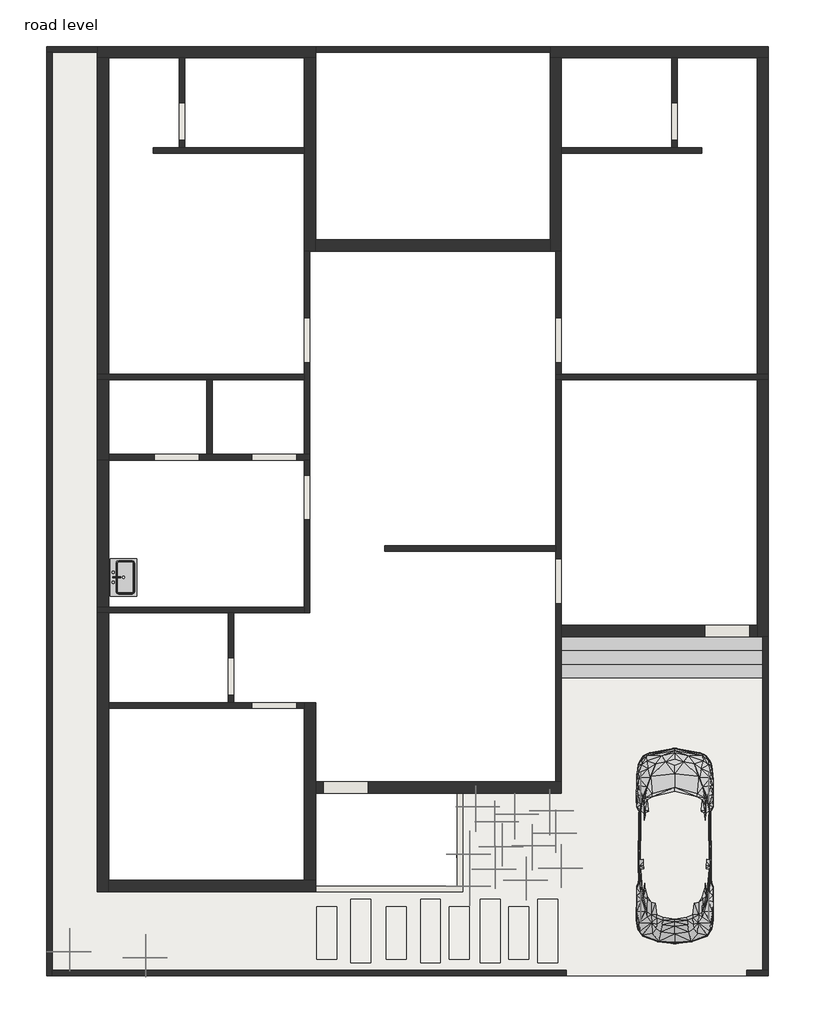
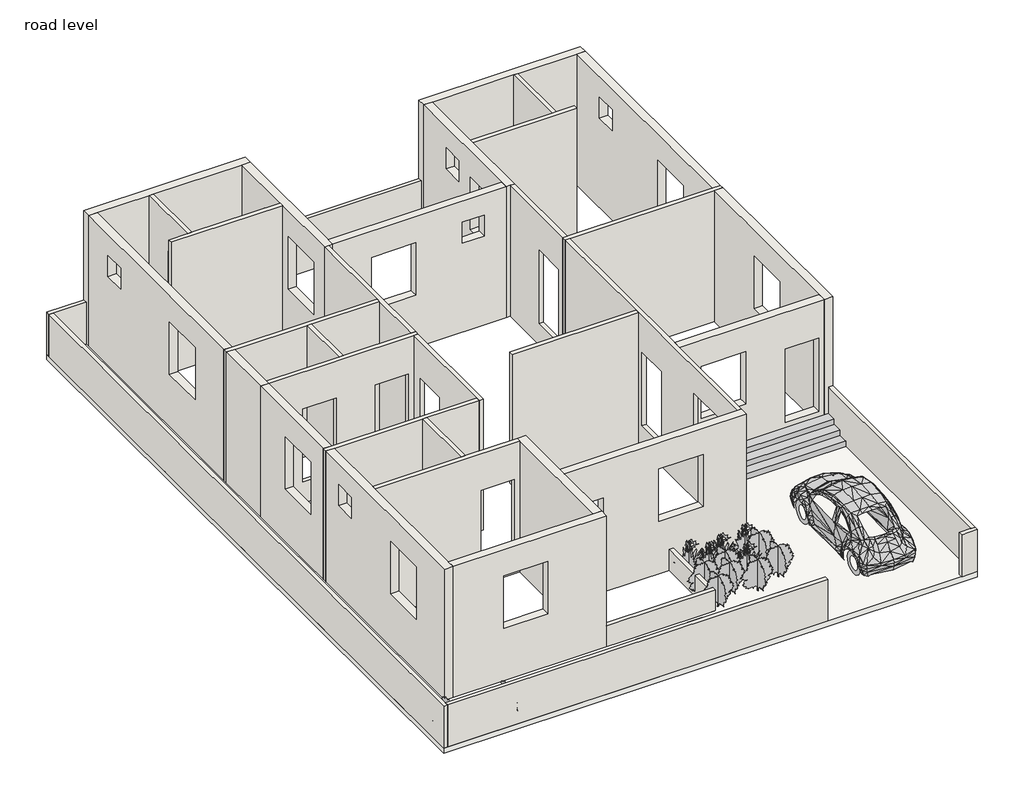
# One storey: 39 walls, 14 geographic elements, 2 slabs, 1 flow terminal, 1 furniture element, 1 proxy.
"""IFC4 building model written with IfcOpenShell, lengths in millimetres."""

from ifc_helpers import new_model, si_unit, frame, origin, origin_with_axes, place, context, project, spatial, polyline, outline, extrude, faceted_brep, transform, mapped, element, save
from components import rpc_beetle_rpc_beetle_31f8b51e, flow_terminal_4d548711, casework_15_casework_15_947a4ada, rpc_plant_tropical_55f6ff97, rpc_plant_tropical_jungle_flame_3_9c4808c2

model = new_model("IFC4")

# Units and contexts
model_context = context("Model", 3, world=origin())
ifc_project = project(units=[si_unit("LENGTHUNIT", "METRE", prefix="MILLI")], contexts=[model_context])

# Site, building, storey
site = spatial("IfcSite", under=ifc_project)
building = spatial("IfcBuilding", under=site)
storey = spatial("IfcBuildingStorey", under=building, Name="road level", Elevation=0.0)

# Proxy
placement = place(None, origin())
rpc_beetle_rpc_beetle_shape = rpc_beetle_rpc_beetle_31f8b51e(model_context)
element("IfcBuildingElementProxy", 1, Name="RPC Beetle : RPC Beetle", ObjectType="RPC Beetle : RPC Beetle", at=placement, inside=storey, context=model_context, shape_type="MappedRepresentation", body=[
    mapped(rpc_beetle_rpc_beetle_shape, transform((12469.3923267, -477.4503076, 0.0), x_axis=(1.0, 0.0, 0.0), y_axis=(0.0, 1.0, 0.0), z_axis=(0.0, 0.0, 1.0))),
])

# Flow terminal
flow_terminal_shape = flow_terminal_4d548711(model_context)
element("IfcFlowTerminal", 2, ObjectType="Sink Kitchen-Single : 30\" x 21\"", at=placement, inside=storey, context=model_context, shape_type="MappedRepresentation", body=[
    mapped(flow_terminal_shape, transform((1244.9377278, 6212.4604519, 0.0), x_axis=(0.0, 1.0, 0.0), y_axis=(-1.0, 0.0, 0.0), z_axis=(0.0, 0.0, 1.0))),
])

# Furniture
casework_15_casework_15_shape = casework_15_casework_15_947a4ada(model_context)
element("IfcFurniture", 3, ObjectType="Casework 15 : Casework 15", at=placement, inside=storey, context=model_context, shape_type="MappedRepresentation", body=[
    mapped(casework_15_casework_15_shape, transform((0.0, 0.0, 0.0), x_axis=(1.0, 0.0, 0.0), y_axis=(0.0, 1.0, 0.0), z_axis=(0.0, 0.0, 1.0))),
])

# Geographic elements
rpc_plant_tropical_shape = rpc_plant_tropical_55f6ff97(model_context)
element("IfcGeographicElement", 4, ObjectType="RPC Plant - Tropical", at=placement, inside=storey, context=model_context, shape_type="MappedRepresentation", body=[
    mapped(rpc_plant_tropical_shape, transform((8418.0923267, 1554.5496924, 0.0), x_axis=(1.0, 0.0, 0.0), y_axis=(0.0, 1.0, 0.0), z_axis=(0.0, 0.0, 1.0))),
])
element("IfcGeographicElement", 5, ObjectType="RPC Plant - Tropical", at=placement, inside=storey, context=model_context, shape_type="MappedRepresentation", body=[
    mapped(rpc_plant_tropical_shape, transform((9205.4923267, 1402.1496924, 0.0), x_axis=(1.0, 0.0, 0.0), y_axis=(0.0, 1.0, 0.0), z_axis=(0.0, 0.0, 1.0))),
])
element("IfcGeographicElement", 6, ObjectType="RPC Plant - Tropical", at=placement, inside=storey, context=model_context, shape_type="MappedRepresentation", body=[
    mapped(rpc_plant_tropical_shape, transform((9916.6923267, 1478.3496924, 0.0), x_axis=(1.0, 0.0, 0.0), y_axis=(0.0, 1.0, 0.0), z_axis=(0.0, 0.0, 1.0))),
])
element("IfcGeographicElement", 7, ObjectType="RPC Plant - Tropical", at=placement, inside=storey, context=model_context, shape_type="MappedRepresentation", body=[
    mapped(rpc_plant_tropical_shape, transform((8799.0923267, 1249.7496924, 0.0), x_axis=(1.0, 0.0, 0.0), y_axis=(0.0, 1.0, 0.0), z_axis=(0.0, 0.0, 1.0))),
])
element("IfcGeographicElement", 8, ObjectType="RPC Plant - Tropical", at=placement, inside=storey, context=model_context, shape_type="MappedRepresentation", body=[
    mapped(rpc_plant_tropical_shape, transform((9561.0923267, 767.1496924, 0.0), x_axis=(1.0, 0.0, 0.0), y_axis=(0.0, 1.0, 0.0), z_axis=(0.0, 0.0, 1.0))),
])
rpc_plant_tropical_jungle_flame_3_shape = rpc_plant_tropical_jungle_flame_3_9c4808c2(model_context)
element("IfcGeographicElement", 9, ObjectType="RPC Plant - Tropical : Jungle Flame - 3'", at=placement, inside=storey, context=model_context, shape_type="MappedRepresentation", body=[
    mapped(rpc_plant_tropical_jungle_flame_3_shape, transform((8291.0923267, 589.3496924, 0.0), x_axis=(1.0, 0.0, 0.0), y_axis=(0.0, 1.0, 0.0), z_axis=(0.0, 0.0, 1.0))),
])
element("IfcGeographicElement", 10, ObjectType="RPC Plant - Tropical : Jungle Flame - 3'", at=placement, inside=storey, context=model_context, shape_type="MappedRepresentation", body=[
    mapped(rpc_plant_tropical_jungle_flame_3_shape, transform((8951.4923267, 741.7496924, 0.0), x_axis=(1.0, 0.0, 0.0), y_axis=(0.0, 1.0, 0.0), z_axis=(0.0, 0.0, 1.0))),
])
element("IfcGeographicElement", 11, ObjectType="RPC Plant - Tropical : Jungle Flame - 3'", at=placement, inside=storey, context=model_context, shape_type="MappedRepresentation", body=[
    mapped(rpc_plant_tropical_jungle_flame_3_shape, transform((10157.9923267, 309.9496924, 0.0), x_axis=(1.0, 0.0, 0.0), y_axis=(0.0, 1.0, 0.0), z_axis=(0.0, 0.0, 1.0))),
])
element("IfcGeographicElement", 12, ObjectType="RPC Plant - Tropical : Jungle Flame - 3'", at=placement, inside=storey, context=model_context, shape_type="MappedRepresentation", body=[
    mapped(rpc_plant_tropical_jungle_flame_3_shape, transform((10043.6923267, 1021.1496924, 0.0), x_axis=(1.0, 0.0, 0.0), y_axis=(0.0, 1.0, 0.0), z_axis=(0.0, 0.0, 1.0))),
])
element("IfcGeographicElement", 13, ObjectType="RPC Plant - Tropical : Jungle Flame - 3'", at=placement, inside=storey, context=model_context, shape_type="MappedRepresentation", body=[
    mapped(rpc_plant_tropical_jungle_flame_3_shape, transform((9446.9910318, 55.9496924, 0.0), x_axis=(1.0, 0.0, 0.0), y_axis=(0.0, 1.0, 0.0), z_axis=(0.0, 0.0, 1.0))),
])
element("IfcGeographicElement", 14, ObjectType="RPC Plant - Tropical : Jungle Flame - 3'", at=placement, inside=storey, context=model_context, shape_type="MappedRepresentation", body=[
    mapped(rpc_plant_tropical_jungle_flame_3_shape, transform((8291.0923267, -58.3503076, 0.0), x_axis=(1.0, 0.0, 0.0), y_axis=(0.0, 1.0, 0.0), z_axis=(0.0, 0.0, 1.0))),
])
element("IfcGeographicElement", 15, ObjectType="RPC Plant - Tropical : Jungle Flame - 3'", at=placement, inside=storey, context=model_context, shape_type="MappedRepresentation", body=[
    mapped(rpc_plant_tropical_jungle_flame_3_shape, transform((8807.0822913, 284.5496924, 0.0), x_axis=(1.0, 0.0, 0.0), y_axis=(0.0, 1.0, 0.0), z_axis=(0.0, 0.0, 1.0))),
])
element("IfcGeographicElement", 16, ObjectType="RPC Plant - Tropical : Jungle Flame - 3'", at=placement, inside=storey, context=model_context, shape_type="MappedRepresentation", body=[
    mapped(rpc_plant_tropical_jungle_flame_3_shape, transform((150.3923267, -1391.8503076, 0.0), x_axis=(1.0, 0.0, 0.0), y_axis=(0.0, 1.0, 0.0), z_axis=(0.0, 0.0, 1.0))),
])
element("IfcGeographicElement", 17, ObjectType="RPC Plant - Tropical : Jungle Flame - 3'", at=placement, inside=storey, context=model_context, shape_type="MappedRepresentation", body=[
    mapped(rpc_plant_tropical_jungle_flame_3_shape, transform((1699.7923267, -1518.8503076, 0.0), x_axis=(1.0, 0.0, 0.0), y_axis=(0.0, 1.0, 0.0), z_axis=(0.0, 0.0, 1.0))),
])

# Slabs
element("IfcSlab", 18, at=placement, inside=storey, context=model_context, shape_type="SweptSolid", body=[
    extrude(outline(polyline([(5586.9696389, -1544.2503076), (5180.5696389, -1544.2503076), (5180.5696389, -477.4503076), (5586.9696389, -477.4503076), (5586.9696389, -1544.2503076)])), frame((0.0, 0.0, -50.8), z_axis=(0.0, 0.0, 1.0), x_axis=(1.0, 0.0, 0.0)), (0.0, 0.0, 1.0), 101.6),
    extrude(outline(polyline([(6276.4251133, -1620.4503076), (5870.0251133, -1620.4503076), (5870.0251133, -325.0503076), (6276.4251133, -325.0503076), (6276.4251133, -1620.4503076)])), frame((0.0, 0.0, -50.8), z_axis=(0.0, 0.0, 1.0), x_axis=(1.0, 0.0, 0.0)), (0.0, 0.0, 1.0), 101.6),
    extrude(outline(polyline([(6999.06314, -1544.2503076), (6592.66314, -1544.2503076), (6592.66314, -477.4503076), (6999.06314, -477.4503076), (6999.06314, -1544.2503076)])), frame((0.0, 0.0, -50.8), z_axis=(0.0, 0.0, 1.0), x_axis=(1.0, 0.0, 0.0)), (0.0, 0.0, 1.0), 101.6),
    extrude(outline(polyline([(7696.9670249, -1620.4503076), (7290.5670249, -1620.4503076), (7290.5670249, -325.0503076), (7696.9670249, -325.0503076), (7696.9670249, -1620.4503076)])), frame((0.0, 0.0, -50.8), z_axis=(0.0, 0.0, 1.0), x_axis=(1.0, 0.0, 0.0)), (0.0, 0.0, 1.0), 101.6),
    extrude(outline(polyline([(8277.6567255, -1544.2503076), (7871.2567255, -1544.2503076), (7871.2567255, -477.4503076), (8277.6567255, -477.4503076), (8277.6567255, -1544.2503076)])), frame((0.0, 0.0, -50.8), z_axis=(0.0, 0.0, 1.0), x_axis=(1.0, 0.0, 0.0)), (0.0, 0.0, 1.0), 101.6),
    extrude(outline(polyline([(8916.1156077, -1620.4503076), (8509.7156077, -1620.4503076), (8509.7156077, -325.0503076), (8916.1156077, -325.0503076), (8916.1156077, -1620.4503076)])), frame((0.0, 0.0, -50.8), z_axis=(0.0, 0.0, 1.0), x_axis=(1.0, 0.0, 0.0)), (0.0, 0.0, 1.0), 101.6),
    extrude(outline(polyline([(9492.8822913, -1544.2503076), (9086.4822913, -1544.2503076), (9086.4822913, -477.4503076), (9492.8822913, -477.4503076), (9492.8822913, -1544.2503076)])), frame((0.0, 0.0, -50.8), z_axis=(0.0, 0.0, 1.0), x_axis=(1.0, 0.0, 0.0)), (0.0, 0.0, 1.0), 101.6),
    extrude(outline(polyline([(10081.9910318, -1620.4503076), (9675.5910318, -1620.4503076), (9675.5910318, -325.0503076), (10081.9910318, -325.0503076), (10081.9910318, -1620.4503076)])), frame((0.0, 0.0, -50.8), z_axis=(0.0, 0.0, 1.0), x_axis=(1.0, 0.0, 0.0)), (0.0, 0.0, 1.0), 101.6),
])
element("IfcSlab", 19, at=placement, inside=storey, context=model_context, shape_type="SweptSolid", body=[
    extrude(outline(polyline([(709.1923267, 17035.8496924), (709.1923267, -172.6503076), (8151.3923267, -172.6503076), (8151.3923267, 1833.9496924), (10157.9923267, 1833.9496924), (10157.9923267, 5021.6496924), (14374.3923267, 5021.6496924), (14374.3923267, -1887.1503076), (-319.5076733, -1887.1503076), (-319.5076733, 17035.8496924), (709.1923267, 17035.8496924)])), frame((0.0, 0.0, -152.4), z_axis=(0.0, 0.0, 1.0), x_axis=(1.0, 0.0, 0.0)), (0.0, 0.0, 1.0), 152.4),
])

# Walls
element("IfcWall", 20, at=placement, inside=storey, context=model_context, shape_type="Brep", body=[
    faceted_brep([(709.1923267, 16807.2496924, 3810.0), (709.1923267, 16807.2496924, 0.0), (937.7923267, 16807.2496924, 0.0), (2372.8923267, 16807.2496924, 0.0), (2487.1923267, 16807.2496924, 0.0), (4925.5923267, 16807.2496924, 0.0), (5154.1923267, 16807.2496924, 0.0), (5154.1923267, 16807.2496924, 3810.0), (4925.5923267, 16807.2496924, 3810.0), (2487.1923267, 16807.2496924, 3810.0), (2372.8923267, 16807.2496924, 3810.0), (937.7923267, 16807.2496924, 3810.0), (709.1923267, 17035.8496924, 0.0), (709.1923267, 17035.8496924, 1219.2), (709.1923267, 17035.8496924, 3810.0), (5154.1923267, 17035.8496924, 3810.0), (5154.1923267, 17035.8496924, 1524.0), (5154.1923267, 17035.8496924, 0.0), (709.1923267, 16921.5496924, 0.0), (5154.1923267, 16921.5496924, 0.0)], [[[0, 1, 2, 3, 4, 5, 6, 7, 8, 9, 10, 11]], [[12, 13, 14, 15, 16, 17]], [[6, 5, 4, 3, 2, 1, 18, 12, 17, 19]], [[0, 11, 10, 9, 8, 7, 15, 14]], [[6, 19, 17, 16, 15, 7]], [[0, 14, 13, 12, 18, 1]]]),
])
element("IfcWall", 21, at=placement, inside=storey, context=model_context, shape_type="Brep", body=[
    faceted_brep([(4925.5923267, 16807.2496924, 3810.0), (4925.5923267, 16807.2496924, 0.0), (4925.5923267, 14978.4496924, 0.0), (4925.5923267, 14864.1496924, 0.0), (4925.5923267, 12870.2496924, 0.0), (4925.5923267, 12870.2496924, 3810.0), (4925.5923267, 14864.1496924, 3810.0), (4925.5923267, 14978.4496924, 3810.0), (4925.5923267, 13390.9496924, 3048.0), (4925.5923267, 13390.9496924, 1524.0), (4925.5923267, 14610.1496924, 1524.0), (4925.5923267, 14610.1496924, 3048.0), (4925.5923267, 15130.8496924, 3200.4), (4925.5923267, 15130.8496924, 2590.8), (4925.5923267, 15740.4496924, 2590.8), (4925.5923267, 15740.4496924, 3200.4), (5154.1923267, 16807.2496924, 0.0), (5154.1923267, 16807.2496924, 3810.0), (5154.1923267, 13098.8496924, 3810.0), (5154.1923267, 12870.2496924, 3810.0), (5154.1923267, 12870.2496924, 0.0), (5154.1923267, 13098.8496924, 0.0), (5154.1923267, 13390.9496924, 3048.0), (5154.1923267, 14610.1496924, 3048.0), (5154.1923267, 14610.1496924, 1524.0), (5154.1923267, 13390.9496924, 1524.0), (5154.1923267, 15130.8496924, 3200.4), (5154.1923267, 15740.4496924, 3200.4), (5154.1923267, 15740.4496924, 2590.8), (5154.1923267, 15130.8496924, 2590.8), (5039.8923267, 12870.2496924, 0.0), (5039.8923267, 12870.2496924, 3810.0)], [[[0, 1, 2, 3, 4, 5, 6, 7], [8, 9, 10, 11], [12, 13, 14, 15]], [[16, 17, 18, 19, 20, 21], [22, 23, 24, 25], [26, 27, 28, 29]], [[4, 3, 2, 1, 16, 21, 20, 30]], [[0, 7, 6, 5, 31, 19, 18, 17]], [[5, 4, 30, 20, 19, 31]], [[9, 8, 22, 25]], [[10, 9, 25, 24]], [[11, 10, 24, 23]], [[8, 11, 23, 22]], [[13, 12, 26, 29]], [[14, 13, 29, 28]], [[15, 14, 28, 27]], [[12, 15, 27, 26]], [[0, 17, 16, 1]]]),
])
element("IfcWall", 22, at=placement, inside=storey, context=model_context, shape_type="Brep", body=[
    faceted_brep([(4925.5923267, 14978.4496924, 0.0), (2487.1923267, 14978.4496924, 0.0), (2372.8923267, 14978.4496924, 0.0), (1852.1923267, 14978.4496924, 0.0), (1852.1923267, 14978.4496924, 3810.0), (2372.8923267, 14978.4496924, 3810.0), (2487.1923267, 14978.4496924, 3810.0), (4925.5923267, 14978.4496924, 3810.0), (4925.5923267, 14864.1496924, 0.0), (4925.5923267, 14864.1496924, 3810.0), (1852.1923267, 14864.1496924, 3810.0), (1852.1923267, 14864.1496924, 0.0)], [[[0, 1, 2, 3, 4, 5, 6, 7]], [[8, 9, 10, 11]], [[3, 2, 1, 0, 8, 11]], [[4, 3, 11, 10]], [[7, 6, 5, 4, 10, 9]], [[0, 7, 9, 8]]]),
])
element("IfcWall", 23, at=placement, inside=storey, context=model_context, shape_type="Brep", body=[
    faceted_brep([(4925.5923267, 10368.3496924, 0.0), (937.7923267, 10368.3496924, 0.0), (709.1923267, 10368.3496924, 0.0), (709.1923267, 10368.3496924, 3810.0), (937.7923267, 10368.3496924, 3810.0), (4925.5923267, 10368.3496924, 3810.0), (4925.5923267, 10254.0496924, 0.0), (4925.5923267, 10254.0496924, 3810.0), (3052.3423267, 10254.0496924, 3810.0), (2938.0423267, 10254.0496924, 3810.0), (937.7923267, 10254.0496924, 3810.0), (709.1923267, 10254.0496924, 3810.0), (709.1923267, 10254.0496924, 0.0), (937.7923267, 10254.0496924, 0.0), (2938.0423267, 10254.0496924, 0.0), (3052.3423267, 10254.0496924, 0.0)], [[[0, 1, 2, 3, 4, 5]], [[6, 7, 8, 9, 10, 11, 12, 13, 14, 15]], [[2, 1, 0, 6, 15, 14, 13, 12]], [[5, 4, 3, 11, 10, 9, 8, 7]], [[0, 5, 7, 6]], [[3, 2, 12, 11]]]),
])
element("IfcWall", 24, at=placement, inside=storey, context=model_context, shape_type="SweptSolid", body=[
    extrude(outline(polyline([(10368.3496924, 0.0), (10368.3496924, 3810.0), (16807.2496924, 3810.0), (16807.2496924, 0.0), (10368.3496924, 0.0)]), holes=[polyline([(12959.1496924, 3048.0), (11739.9496924, 3048.0), (11739.9496924, 1524.0), (12959.1496924, 1524.0), (12959.1496924, 3048.0)]), polyline([(15892.8496924, 3200.4), (15283.2496924, 3200.4), (15283.2496924, 2590.8), (15892.8496924, 2590.8), (15892.8496924, 3200.4)])]), frame((709.1923267, 0.0, 0.0), z_axis=(1.0, 0.0, 0.0), x_axis=(0.0, 1.0, 0.0)), (0.0, 0.0, 1.0), 228.6),
])
element("IfcWall", 25, at=placement, inside=storey, context=model_context, shape_type="Brep", body=[
    faceted_brep([(9929.3923267, 16807.2496924, 3810.0), (9929.3923267, 16807.2496924, 0.0), (10157.9923267, 16807.2496924, 0.0), (12405.8923267, 16807.2496924, 0.0), (12520.1923267, 16807.2496924, 0.0), (14145.7923267, 16807.2496924, 0.0), (14374.3923267, 16807.2496924, 0.0), (14374.3923267, 16807.2496924, 3810.0), (14145.7923267, 16807.2496924, 3810.0), (12520.1923267, 16807.2496924, 3810.0), (12405.8923267, 16807.2496924, 3810.0), (10157.9923267, 16807.2496924, 3810.0), (9929.3923267, 17035.8496924, 0.0), (9929.3923267, 17035.8496924, 1524.0), (9929.3923267, 17035.8496924, 3810.0), (14374.3923267, 17035.8496924, 3810.0), (14374.3923267, 17035.8496924, 0.0), (9929.3923267, 16921.5496924, 0.0)], [[[0, 1, 2, 3, 4, 5, 6, 7, 8, 9, 10, 11]], [[12, 13, 14, 15, 16]], [[6, 5, 4, 3, 2, 1, 17, 12, 16]], [[0, 11, 10, 9, 8, 7, 15, 14]], [[7, 6, 16, 15]], [[0, 14, 13, 12, 17, 1]]]),
])
element("IfcWall", 26, at=placement, inside=storey, context=model_context, shape_type="Brep", body=[
    faceted_brep([(9929.3923267, 16807.2496924, 3810.0), (9929.3923267, 16807.2496924, 0.0), (9929.3923267, 13098.8496924, 0.0), (9929.3923267, 12870.2496924, 0.0), (9929.3923267, 12870.2496924, 3810.0), (9929.3923267, 13098.8496924, 3810.0), (9929.3923267, 14591.0996924, 3048.0), (9929.3923267, 13371.8996924, 3048.0), (9929.3923267, 13371.8996924, 1524.0), (9929.3923267, 14591.0996924, 1524.0), (9929.3923267, 15740.4496924, 3200.4), (9929.3923267, 15130.8496924, 3200.4), (9929.3923267, 15130.8496924, 2590.8), (9929.3923267, 15740.4496924, 2590.8), (10157.9923267, 16807.2496924, 0.0), (10157.9923267, 16807.2496924, 3810.0), (10157.9923267, 14978.4496924, 3810.0), (10157.9923267, 14864.1496924, 3810.0), (10157.9923267, 12870.2496924, 3810.0), (10157.9923267, 12870.2496924, 0.0), (10157.9923267, 14864.1496924, 0.0), (10157.9923267, 14978.4496924, 0.0), (10157.9923267, 14591.0996924, 3048.0), (10157.9923267, 14591.0996924, 1524.0), (10157.9923267, 13371.8996924, 1524.0), (10157.9923267, 13371.8996924, 3048.0), (10157.9923267, 15740.4496924, 3200.4), (10157.9923267, 15740.4496924, 2590.8), (10157.9923267, 15130.8496924, 2590.8), (10157.9923267, 15130.8496924, 3200.4), (10043.6923267, 12870.2496924, 0.0), (10043.6923267, 12870.2496924, 3810.0)], [[[0, 1, 2, 3, 4, 5], [6, 7, 8, 9], [10, 11, 12, 13]], [[14, 15, 16, 17, 18, 19, 20, 21], [22, 23, 24, 25], [26, 27, 28, 29]], [[3, 2, 1, 14, 21, 20, 19, 30]], [[0, 5, 4, 31, 18, 17, 16, 15]], [[4, 3, 30, 19, 18, 31]], [[23, 22, 6, 9]], [[24, 23, 9, 8]], [[25, 24, 8, 7]], [[22, 25, 7, 6]], [[27, 26, 10, 13]], [[28, 27, 13, 12]], [[29, 28, 12, 11]], [[26, 29, 11, 10]], [[0, 15, 14, 1]]]),
])
element("IfcWall", 27, at=placement, inside=storey, context=model_context, shape_type="Brep", body=[
    faceted_brep([(10157.9923267, 14864.1496924, 0.0), (13015.4923267, 14864.1496924, 0.0), (13015.4923267, 14864.1496924, 3810.0), (10157.9923267, 14864.1496924, 3810.0), (10157.9923267, 14978.4496924, 0.0), (10157.9923267, 14978.4496924, 3810.0), (12405.8923267, 14978.4496924, 3810.0), (12520.1923267, 14978.4496924, 3810.0), (13015.4923267, 14978.4496924, 3810.0), (13015.4923267, 14978.4496924, 0.0), (12520.1923267, 14978.4496924, 0.0), (12405.8923267, 14978.4496924, 0.0)], [[[0, 1, 2, 3]], [[4, 5, 6, 7, 8, 9, 10, 11]], [[1, 0, 4, 11, 10, 9]], [[2, 1, 9, 8]], [[3, 2, 8, 7, 6, 5]], [[0, 3, 5, 4]]]),
])
element("IfcWall", 28, at=placement, inside=storey, context=model_context, shape_type="Brep", body=[
    faceted_brep([(4925.5923267, 12870.2496924, 0.0), (4925.5923267, 10368.3496924, 0.0), (4925.5923267, 10254.0496924, 0.0), (4925.5923267, 8730.0496924, 0.0), (4925.5923267, 8730.0496924, 3810.0), (4925.5923267, 10254.0496924, 3810.0), (4925.5923267, 10368.3496924, 3810.0), (4925.5923267, 12870.2496924, 3810.0), (4925.5923267, 11511.3496924, 609.6), (4925.5923267, 11511.3496924, 2743.2), (4925.5923267, 10596.9496924, 2743.2), (4925.5923267, 10596.9496924, 609.6), (5039.8923267, 12870.2496924, 0.0), (5039.8923267, 12870.2496924, 3810.0), (5039.8923267, 8730.0496924, 3810.0), (5039.8923267, 8730.0496924, 0.0), (5039.8923267, 11511.3496924, 609.6), (5039.8923267, 10596.9496924, 609.6), (5039.8923267, 10596.9496924, 2743.2), (5039.8923267, 11511.3496924, 2743.2)], [[[0, 1, 2, 3, 4, 5, 6, 7], [8, 9, 10, 11]], [[12, 13, 14, 15], [16, 17, 18, 19]], [[3, 2, 1, 0, 12, 15]], [[7, 6, 5, 4, 14, 13]], [[0, 7, 13, 12]], [[4, 3, 15, 14]], [[17, 16, 8, 11]], [[18, 17, 11, 10]], [[19, 18, 10, 9]], [[16, 19, 9, 8]]]),
])
element("IfcWall", 29, at=placement, inside=storey, context=model_context, shape_type="SweptSolid", body=[
    extrude(outline(polyline([(0.0, 9929.3923267), (3810.0, 9929.3923267), (3810.0, 5154.1923267), (0.0, 5154.1923267), (0.0, 9929.3923267)]), holes=[polyline([(3048.0, 7440.1923267), (1524.0, 7440.1923267), (1524.0, 6220.9923267), (3048.0, 6220.9923267), (3048.0, 7440.1923267)]), polyline([(3200.4, 9319.7923267), (2590.8, 9319.7923267), (2590.8, 8710.1923267), (3200.4, 8710.1923267), (3200.4, 9319.7923267)])]), frame((0.0, 12870.2496924, 0.0), z_axis=(0.0, 1.0, 0.0), x_axis=(0.0, 0.0, 1.0)), (0.0, 0.0, 1.0), 228.6),
])
element("IfcWall", 30, at=placement, inside=storey, context=model_context, shape_type="Brep", body=[
    faceted_brep([(10043.6923267, 10254.0496924, 0.0), (10157.9923267, 10254.0496924, 0.0), (14145.7923267, 10254.0496924, 0.0), (14374.3923267, 10254.0496924, 0.0), (14374.3923267, 10254.0496924, 3810.0), (14145.7923267, 10254.0496924, 3810.0), (10157.9923267, 10254.0496924, 3810.0), (10043.6923267, 10254.0496924, 3810.0), (10043.6923267, 10368.3496924, 0.0), (10043.6923267, 10368.3496924, 3810.0), (10157.9923267, 10368.3496924, 3810.0), (14145.7923267, 10368.3496924, 3810.0), (14374.3923267, 10368.3496924, 3810.0), (14374.3923267, 10368.3496924, 0.0), (14145.7923267, 10368.3496924, 0.0), (10157.9923267, 10368.3496924, 0.0)], [[[0, 1, 2, 3, 4, 5, 6, 7]], [[8, 9, 10, 11, 12, 13, 14, 15]], [[3, 2, 1, 0, 8, 15, 14, 13]], [[7, 6, 5, 4, 12, 11, 10, 9]], [[4, 3, 13, 12]], [[0, 7, 9, 8]]]),
])
element("IfcWall", 31, at=placement, inside=storey, context=model_context, shape_type="SweptSolid", body=[
    extrude(outline(polyline([(10368.3496924, 0.0), (10368.3496924, 3810.0), (16807.2496924, 3810.0), (16807.2496924, 0.0), (10368.3496924, 0.0)]), holes=[polyline([(11739.9496924, 3048.0), (11739.9496924, 1524.0), (12959.1496924, 1524.0), (12959.1496924, 3048.0), (11739.9496924, 3048.0)]), polyline([(15130.8496924, 3200.4), (15130.8496924, 2590.8), (15740.4496924, 2590.8), (15740.4496924, 3200.4), (15130.8496924, 3200.4)])]), frame((14145.7923267, 0.0, 0.0), z_axis=(1.0, 0.0, 0.0), x_axis=(0.0, 1.0, 0.0)), (0.0, 0.0, 1.0), 228.6),
])
element("IfcWall", 32, at=placement, inside=storey, context=model_context, shape_type="Brep", body=[
    faceted_brep([(709.1923267, 10254.0496924, 0.0), (709.1923267, 8615.7496924, 0.0), (709.1923267, 8615.7496924, 3810.0), (709.1923267, 10254.0496924, 3810.0), (937.7923267, 10254.0496924, 0.0), (937.7923267, 10254.0496924, 3810.0), (937.7923267, 8730.0496924, 3810.0), (937.7923267, 8615.7496924, 3810.0), (937.7923267, 8615.7496924, 0.0), (937.7923267, 8730.0496924, 0.0)], [[[0, 1, 2, 3]], [[4, 5, 6, 7, 8, 9]], [[1, 0, 4, 9, 8]], [[3, 2, 7, 6, 5]], [[0, 3, 5, 4]], [[2, 1, 8, 7]]]),
])
element("IfcWall", 33, at=placement, inside=storey, context=model_context, shape_type="Brep", body=[
    faceted_brep([(937.7923267, 8615.7496924, 0.0), (4925.5923267, 8615.7496924, 0.0), (5039.8923267, 8615.7496924, 0.0), (5039.8923267, 8615.7496924, 3810.0), (4925.5923267, 8615.7496924, 3810.0), (937.7923267, 8615.7496924, 3810.0), (1871.2423267, 8615.7496924, 609.6), (1871.2423267, 8615.7496924, 2743.2), (2785.6423267, 8615.7496924, 2743.2), (2785.6423267, 8615.7496924, 609.6), (3858.7923267, 8615.7496924, 609.6), (3858.7923267, 8615.7496924, 2743.2), (4773.1923267, 8615.7496924, 2743.2), (4773.1923267, 8615.7496924, 609.6), (937.7923267, 8730.0496924, 0.0), (937.7923267, 8730.0496924, 3810.0), (2938.0423267, 8730.0496924, 3810.0), (3052.3423267, 8730.0496924, 3810.0), (4925.5923267, 8730.0496924, 3810.0), (5039.8923267, 8730.0496924, 3810.0), (5039.8923267, 8730.0496924, 0.0), (4925.5923267, 8730.0496924, 0.0), (3052.3423267, 8730.0496924, 0.0), (2938.0423267, 8730.0496924, 0.0), (1871.2423267, 8730.0496924, 609.6), (2785.6423267, 8730.0496924, 609.6), (2785.6423267, 8730.0496924, 2743.2), (1871.2423267, 8730.0496924, 2743.2), (3858.7923267, 8730.0496924, 609.6), (4773.1923267, 8730.0496924, 609.6), (4773.1923267, 8730.0496924, 2743.2), (3858.7923267, 8730.0496924, 2743.2)], [[[0, 1, 2, 3, 4, 5], [6, 7, 8, 9], [10, 11, 12, 13]], [[14, 15, 16, 17, 18, 19, 20, 21, 22, 23], [24, 25, 26, 27], [28, 29, 30, 31]], [[2, 1, 0, 14, 23, 22, 21, 20]], [[5, 4, 3, 19, 18, 17, 16, 15]], [[0, 5, 15, 14]], [[3, 2, 20, 19]], [[25, 24, 6, 9]], [[26, 25, 9, 8]], [[27, 26, 8, 7]], [[24, 27, 7, 6]], [[29, 28, 10, 13]], [[30, 29, 13, 12]], [[31, 30, 12, 11]], [[28, 31, 11, 10]]]),
])
element("IfcWall", 34, at=placement, inside=storey, context=model_context, shape_type="Brep", body=[
    faceted_brep([(4925.5923267, 8615.7496924, 0.0), (4925.5923267, 5618.5496924, 0.0), (4925.5923267, 5504.2496924, 0.0), (4925.5923267, 5504.2496924, 3810.0), (4925.5923267, 5618.5496924, 3810.0), (4925.5923267, 8615.7496924, 3810.0), (4925.5923267, 7396.5496924, 609.6), (4925.5923267, 8310.9496924, 609.6), (4925.5923267, 8310.9496924, 2743.2), (4925.5923267, 7396.5496924, 2743.2), (5039.8923267, 8615.7496924, 0.0), (5039.8923267, 8615.7496924, 3810.0), (5039.8923267, 5504.2496924, 3810.0), (5039.8923267, 5504.2496924, 0.0), (5039.8923267, 7396.5496924, 609.6), (5039.8923267, 7396.5496924, 2743.2), (5039.8923267, 8310.9496924, 2743.2), (5039.8923267, 8310.9496924, 609.6)], [[[0, 1, 2, 3, 4, 5], [6, 7, 8, 9]], [[10, 11, 12, 13], [14, 15, 16, 17]], [[2, 1, 0, 10, 13]], [[5, 4, 3, 12, 11]], [[0, 5, 11, 10]], [[3, 2, 13, 12]], [[7, 6, 14, 17]], [[8, 7, 17, 16]], [[9, 8, 16, 15]], [[6, 9, 15, 14]]]),
])
element("IfcWall", 35, at=placement, inside=storey, context=model_context, shape_type="Brep", body=[
    faceted_brep([(4925.5923267, 5618.5496924, 0.0), (937.7923267, 5618.5496924, 0.0), (709.1923267, 5618.5496924, 0.0), (709.1923267, 5618.5496924, 3810.0), (937.7923267, 5618.5496924, 3810.0), (4925.5923267, 5618.5496924, 3810.0), (4925.5923267, 5504.2496924, 0.0), (4925.5923267, 5504.2496924, 3810.0), (3490.4923267, 5504.2496924, 3810.0), (3376.1923267, 5504.2496924, 3810.0), (937.7923267, 5504.2496924, 3810.0), (709.1923267, 5504.2496924, 3810.0), (709.1923267, 5504.2496924, 0.0), (937.7923267, 5504.2496924, 0.0), (3376.1923267, 5504.2496924, 0.0), (3490.4923267, 5504.2496924, 0.0)], [[[0, 1, 2, 3, 4, 5]], [[6, 7, 8, 9, 10, 11, 12, 13, 14, 15]], [[2, 1, 0, 6, 15, 14, 13, 12]], [[5, 4, 3, 11, 10, 9, 8, 7]], [[0, 5, 7, 6]], [[3, 2, 12, 11]]]),
])
element("IfcWall", 36, at=placement, inside=storey, context=model_context, shape_type="SweptSolid", body=[
    extrude(outline(polyline([(5618.5496924, 0.0), (5618.5496924, 3810.0), (8615.7496924, 3810.0), (8615.7496924, 0.0), (5618.5496924, 0.0)]), holes=[polyline([(7447.3496924, 3048.0), (6228.1496924, 3048.0), (6228.1496924, 1524.0), (7447.3496924, 1524.0), (7447.3496924, 3048.0)])]), frame((709.1923267, 0.0, 0.0), z_axis=(1.0, 0.0, 0.0), x_axis=(0.0, 1.0, 0.0)), (0.0, 0.0, 1.0), 228.6),
])
element("IfcWall", 37, at=placement, inside=storey, context=model_context, shape_type="SweptSolid", body=[
    extrude(outline(polyline([(3052.3423267, 10254.0496924), (3052.3423267, 8730.0496924), (2938.0423267, 8730.0496924), (2938.0423267, 10254.0496924), (3052.3423267, 10254.0496924)])), origin_with_axes(), (0.0, 0.0, 1.0), 3810.0),
])
element("IfcWall", 38, at=placement, inside=storey, context=model_context, shape_type="SweptSolid", body=[
    extrude(outline(polyline([(12870.2496924, 0.0), (10368.3496924, 0.0), (10368.3496924, 3810.0), (12870.2496924, 3810.0), (12870.2496924, 0.0)]), holes=[polyline([(11511.3496924, 609.6), (11511.3496924, 2743.2), (10596.9496924, 2743.2), (10596.9496924, 609.6), (11511.3496924, 609.6)])]), frame((10043.6923267, 0.0, 0.0), z_axis=(1.0, 0.0, 0.0), x_axis=(0.0, 1.0, 0.0)), (0.0, 0.0, 1.0), 114.3),
])
element("IfcWall", 39, at=placement, inside=storey, context=model_context, shape_type="Brep", body=[
    faceted_brep([(709.1923267, 5504.2496924, 0.0), (709.1923267, -172.6503076, 0.0), (709.1923267, -172.6503076, 3810.0), (709.1923267, 5504.2496924, 3810.0), (709.1923267, 4894.6496924, 3200.4), (709.1923267, 4285.0496924, 3200.4), (709.1923267, 4285.0496924, 2590.8), (709.1923267, 4894.6496924, 2590.8), (709.1923267, 2418.1496924, 3048.0), (709.1923267, 1198.9496924, 3048.0), (709.1923267, 1198.9496924, 1524.0), (709.1923267, 2418.1496924, 1524.0), (937.7923267, 5504.2496924, 0.0), (937.7923267, 5504.2496924, 3810.0), (937.7923267, 3675.4496924, 3810.0), (937.7923267, 3561.1496924, 3810.0), (937.7923267, 55.9496924, 3810.0), (937.7923267, -172.6503076, 3810.0), (937.7923267, -172.6503076, 0.0), (937.7923267, 55.9496924, 0.0), (937.7923267, 3561.1496924, 0.0), (937.7923267, 3675.4496924, 0.0), (937.7923267, 4894.6496924, 3200.4), (937.7923267, 4894.6496924, 2590.8), (937.7923267, 4285.0496924, 2590.8), (937.7923267, 4285.0496924, 3200.4), (937.7923267, 2418.1496924, 3048.0), (937.7923267, 2418.1496924, 1524.0), (937.7923267, 1198.9496924, 1524.0), (937.7923267, 1198.9496924, 3048.0)], [[[0, 1, 2, 3], [4, 5, 6, 7], [8, 9, 10, 11]], [[12, 13, 14, 15, 16, 17, 18, 19, 20, 21], [22, 23, 24, 25], [26, 27, 28, 29]], [[1, 0, 12, 21, 20, 19, 18]], [[3, 2, 17, 16, 15, 14, 13]], [[0, 3, 13, 12]], [[2, 1, 18, 17]], [[23, 22, 4, 7]], [[24, 23, 7, 6]], [[25, 24, 6, 5]], [[22, 25, 5, 4]], [[27, 26, 8, 11]], [[28, 27, 11, 10]], [[29, 28, 10, 9]], [[26, 29, 9, 8]]]),
])
element("IfcWall", 40, at=placement, inside=storey, context=model_context, shape_type="Brep", body=[
    faceted_brep([(937.7923267, 3561.1496924, 0.0), (4925.5923267, 3561.1496924, 0.0), (4925.5923267, 3561.1496924, 3810.0), (937.7923267, 3561.1496924, 3810.0), (3858.7923267, 3561.1496924, 609.6), (3858.7923267, 3561.1496924, 2743.2), (4773.1923267, 3561.1496924, 2743.2), (4773.1923267, 3561.1496924, 609.6), (937.7923267, 3675.4496924, 0.0), (937.7923267, 3675.4496924, 3810.0), (3376.1923267, 3675.4496924, 3810.0), (3490.4923267, 3675.4496924, 3810.0), (4925.5923267, 3675.4496924, 3810.0), (4925.5923267, 3675.4496924, 0.0), (3490.4923267, 3675.4496924, 0.0), (3376.1923267, 3675.4496924, 0.0), (3858.7923267, 3675.4496924, 609.6), (4773.1923267, 3675.4496924, 609.6), (4773.1923267, 3675.4496924, 2743.2), (3858.7923267, 3675.4496924, 2743.2)], [[[0, 1, 2, 3], [4, 5, 6, 7]], [[8, 9, 10, 11, 12, 13, 14, 15], [16, 17, 18, 19]], [[1, 0, 8, 15, 14, 13]], [[3, 2, 12, 11, 10, 9]], [[0, 3, 9, 8]], [[2, 1, 13, 12]], [[17, 16, 4, 7]], [[18, 17, 7, 6]], [[19, 18, 6, 5]], [[16, 19, 5, 4]]]),
])
element("IfcWall", 41, at=placement, inside=storey, context=model_context, shape_type="Brep", body=[
    faceted_brep([(937.7923267, -172.6503076, 0.0), (5154.1923267, -172.6503076, 0.0), (5154.1923267, -172.6503076, 609.6), (5154.1923267, -172.6503076, 3810.0), (937.7923267, -172.6503076, 3810.0), (2322.0923267, -172.6503076, 3048.0), (3541.2923267, -172.6503076, 3048.0), (3541.2923267, -172.6503076, 1524.0), (2322.0923267, -172.6503076, 1524.0), (937.7923267, 55.9496924, 0.0), (937.7923267, 55.9496924, 3810.0), (4925.5923267, 55.9496924, 3810.0), (5154.1923267, 55.9496924, 3810.0), (5154.1923267, 55.9496924, 0.0), (4925.5923267, 55.9496924, 0.0), (2322.0923267, 55.9496924, 3048.0), (2322.0923267, 55.9496924, 1524.0), (3541.2923267, 55.9496924, 1524.0), (3541.2923267, 55.9496924, 3048.0), (5154.1923267, -58.3503076, 0.0)], [[[0, 1, 2, 3, 4], [5, 6, 7, 8]], [[9, 10, 11, 12, 13, 14], [15, 16, 17, 18]], [[1, 0, 9, 14, 13, 19]], [[4, 3, 12, 11, 10]], [[0, 4, 10, 9]], [[16, 15, 5, 8]], [[17, 16, 8, 7]], [[18, 17, 7, 6]], [[15, 18, 6, 5]], [[1, 19, 13, 12, 3, 2]]]),
])
element("IfcWall", 42, at=placement, inside=storey, context=model_context, shape_type="Brep", body=[
    faceted_brep([(5154.1923267, 55.9496924, 3810.0), (5154.1923267, 55.9496924, 0.0), (5154.1923267, 1833.9496924, 0.0), (5154.1923267, 2062.5496924, 0.0), (5154.1923267, 3675.4496924, 0.0), (5154.1923267, 3675.4496924, 3810.0), (5154.1923267, 2062.5496924, 3810.0), (5154.1923267, 1833.9496924, 3810.0), (4925.5923267, 55.9496924, 0.0), (4925.5923267, 55.9496924, 3810.0), (4925.5923267, 3561.1496924, 3810.0), (4925.5923267, 3675.4496924, 3810.0), (4925.5923267, 3675.4496924, 0.0), (4925.5923267, 3561.1496924, 0.0)], [[[0, 1, 2, 3, 4, 5, 6, 7]], [[8, 9, 10, 11, 12, 13]], [[4, 3, 2, 1, 8, 13, 12]], [[0, 7, 6, 5, 11, 10, 9]], [[5, 4, 12, 11]], [[0, 9, 8, 1]]]),
])
element("IfcWall", 43, at=placement, inside=storey, context=model_context, shape_type="Brep", body=[
    faceted_brep([(14145.7923267, 10254.0496924, 0.0), (14145.7923267, 5250.2496924, 0.0), (14145.7923267, 5021.6496924, 0.0), (14145.7923267, 5021.6496924, 3810.0), (14145.7923267, 5250.2496924, 3810.0), (14145.7923267, 10254.0496924, 3810.0), (14145.7923267, 7142.5496924, 3048.0), (14145.7923267, 7142.5496924, 1524.0), (14145.7923267, 8361.7496924, 1524.0), (14145.7923267, 8361.7496924, 3048.0), (14374.3923267, 10254.0496924, 0.0), (14374.3923267, 10254.0496924, 3810.0), (14374.3923267, 5021.6496924, 3810.0), (14374.3923267, 5021.6496924, 1219.2), (14374.3923267, 5021.6496924, 0.0), (14374.3923267, 7142.5496924, 3048.0), (14374.3923267, 8361.7496924, 3048.0), (14374.3923267, 8361.7496924, 1524.0), (14374.3923267, 7142.5496924, 1524.0), (14260.0923267, 5021.6496924, 0.0)], [[[0, 1, 2, 3, 4, 5], [6, 7, 8, 9]], [[10, 11, 12, 13, 14], [15, 16, 17, 18]], [[2, 1, 0, 10, 14, 19]], [[5, 4, 3, 12, 11]], [[0, 5, 11, 10]], [[7, 6, 15, 18]], [[8, 7, 18, 17]], [[9, 8, 17, 16]], [[6, 9, 16, 15]], [[2, 19, 14, 13, 12, 3]]]),
])
element("IfcWall", 44, at=placement, inside=storey, context=model_context, shape_type="SweptSolid", body=[
    extrude(outline(polyline([(0.0, 14145.7923267), (3810.0, 14145.7923267), (3810.0, 10157.9923267), (0.0, 10157.9923267), (0.0, 14145.7923267)]), holes=[polyline([(609.6, 13078.9923267), (2743.2, 13078.9923267), (2743.2, 13993.3923267), (609.6, 13993.3923267), (609.6, 13078.9923267)]), polyline([(3048.0, 10767.5923267), (3048.0, 11986.7923267), (1524.0, 11986.7923267), (1524.0, 10767.5923267), (3048.0, 10767.5923267)])]), frame((0.0, 5021.6496924, 0.0), z_axis=(0.0, 1.0, 0.0), x_axis=(0.0, 0.0, 1.0)), (0.0, 0.0, 1.0), 228.6),
])
element("IfcWall", 45, at=placement, inside=storey, context=model_context, shape_type="Brep", body=[
    faceted_brep([(10157.9923267, 2062.5496924, 0.0), (10157.9923267, 5021.6496924, 0.0), (10157.9923267, 5250.2496924, 0.0), (10157.9923267, 10254.0496924, 0.0), (10157.9923267, 10254.0496924, 3810.0), (10157.9923267, 5250.2496924, 3810.0), (10157.9923267, 5021.6496924, 3810.0), (10157.9923267, 2062.5496924, 3810.0), (10157.9923267, 5694.7496924, 609.6), (10157.9923267, 5694.7496924, 2743.2), (10157.9923267, 6609.1496924, 2743.2), (10157.9923267, 6609.1496924, 609.6), (10157.9923267, 2926.1496924, 3048.0), (10157.9923267, 4145.3496924, 3048.0), (10157.9923267, 4145.3496924, 1524.0), (10157.9923267, 2926.1496924, 1524.0), (10043.6923267, 2062.5496924, 0.0), (10043.6923267, 2062.5496924, 3810.0), (10043.6923267, 6761.5496924, 3810.0), (10043.6923267, 6875.8496924, 3810.0), (10043.6923267, 10254.0496924, 3810.0), (10043.6923267, 10254.0496924, 0.0), (10043.6923267, 6875.8496924, 0.0), (10043.6923267, 6761.5496924, 0.0), (10043.6923267, 5694.7496924, 609.6), (10043.6923267, 6609.1496924, 609.6), (10043.6923267, 6609.1496924, 2743.2), (10043.6923267, 5694.7496924, 2743.2), (10043.6923267, 2926.1496924, 3048.0), (10043.6923267, 2926.1496924, 1524.0), (10043.6923267, 4145.3496924, 1524.0), (10043.6923267, 4145.3496924, 3048.0)], [[[0, 1, 2, 3, 4, 5, 6, 7], [8, 9, 10, 11], [12, 13, 14, 15]], [[16, 17, 18, 19, 20, 21, 22, 23], [24, 25, 26, 27], [28, 29, 30, 31]], [[3, 2, 1, 0, 16, 23, 22, 21]], [[7, 6, 5, 4, 20, 19, 18, 17]], [[0, 7, 17, 16]], [[4, 3, 21, 20]], [[25, 24, 8, 11]], [[26, 25, 11, 10]], [[27, 26, 10, 9]], [[24, 27, 9, 8]], [[29, 28, 12, 15]], [[30, 29, 15, 14]], [[31, 30, 14, 13]], [[28, 31, 13, 12]]]),
])
element("IfcWall", 46, at=placement, inside=storey, context=model_context, shape_type="SweptSolid", body=[
    extrude(outline(polyline([(6563.8923267, 6875.8496924), (10043.6923267, 6875.8496924), (10043.6923267, 6761.5496924), (6563.8923267, 6761.5496924), (6563.8923267, 6875.8496924)])), origin_with_axes(), (0.0, 0.0, 1.0), 3810.0),
])
element("IfcWall", 47, at=placement, inside=storey, context=model_context, shape_type="Brep", body=[
    faceted_brep([(5154.1923267, 1833.9496924, 0.0), (8037.0923267, 1833.9496924, 0.0), (8151.3923267, 1833.9496924, 0.0), (10157.9923267, 1833.9496924, 0.0), (10157.9923267, 1833.9496924, 3810.0), (5154.1923267, 1833.9496924, 3810.0), (6220.9923267, 1833.9496924, 609.6), (5306.5923267, 1833.9496924, 609.6), (5306.5923267, 1833.9496924, 2743.2), (6220.9923267, 1833.9496924, 2743.2), (7757.6923267, 1833.9496924, 3048.0), (8976.8923267, 1833.9496924, 3048.0), (8976.8923267, 1833.9496924, 1524.0), (7757.6923267, 1833.9496924, 1524.0), (5154.1923267, 2062.5496924, 0.0), (5154.1923267, 2062.5496924, 3810.0), (10043.6923267, 2062.5496924, 3810.0), (10157.9923267, 2062.5496924, 3810.0), (10157.9923267, 2062.5496924, 0.0), (10043.6923267, 2062.5496924, 0.0), (6220.9923267, 2062.5496924, 609.6), (6220.9923267, 2062.5496924, 2743.2), (5306.5923267, 2062.5496924, 2743.2), (5306.5923267, 2062.5496924, 609.6), (7757.6923267, 2062.5496924, 3048.0), (7757.6923267, 2062.5496924, 1524.0), (8976.8923267, 2062.5496924, 1524.0), (8976.8923267, 2062.5496924, 3048.0)], [[[0, 1, 2, 3, 4, 5], [6, 7, 8, 9], [10, 11, 12, 13]], [[14, 15, 16, 17, 18, 19], [20, 21, 22, 23], [24, 25, 26, 27]], [[3, 2, 1, 0, 14, 19, 18]], [[5, 4, 17, 16, 15]], [[4, 3, 18, 17]], [[0, 5, 15, 14]], [[7, 6, 20, 23]], [[8, 7, 23, 22]], [[9, 8, 22, 21]], [[6, 9, 21, 20]], [[25, 24, 10, 13]], [[26, 25, 13, 12]], [[27, 26, 12, 11]], [[24, 27, 11, 10]]]),
])
element("IfcWall", 48, at=placement, inside=storey, context=model_context, shape_type="SweptSolid", body=[
    extrude(outline(polyline([(14260.0923267, -1772.8503076), (14260.0923267, 5021.6496924), (14374.3923267, 5021.6496924), (14374.3923267, -1772.8503076), (14260.0923267, -1772.8503076)])), origin_with_axes(), (0.0, 0.0, 1.0), 1219.2),
])
element("IfcWall", 49, at=placement, inside=storey, context=model_context, shape_type="Brep", body=[
    faceted_brep([(709.1923267, 17035.8496924, 0.0), (-319.5076733, 17035.8496924, 0.0), (-319.5076733, 17035.8496924, 1219.2), (709.1923267, 17035.8496924, 1219.2), (709.1923267, 16921.5496924, 0.0), (709.1923267, 16921.5496924, 1219.2), (-205.2076733, 16921.5496924, 1219.2), (-319.5076733, 16921.5496924, 1219.2), (-319.5076733, 16921.5496924, 0.0), (-205.2076733, 16921.5496924, 0.0)], [[[0, 1, 2, 3]], [[4, 5, 6, 7, 8, 9]], [[1, 0, 4, 9, 8]], [[3, 2, 7, 6, 5]], [[0, 3, 5, 4]], [[2, 1, 8, 7]]]),
])
element("IfcWall", 50, at=placement, inside=storey, context=model_context, shape_type="Brep", body=[
    faceted_brep([(-319.5076733, 16921.5496924, 0.0), (-319.5076733, -1887.1503076, 0.0), (-319.5076733, -1887.1503076, 1219.2), (-319.5076733, 16921.5496924, 1219.2), (-205.2076733, 16921.5496924, 0.0), (-205.2076733, 16921.5496924, 1219.2), (-205.2076733, -1772.8503076, 1219.2), (-205.2076733, -1887.1503076, 1219.2), (-205.2076733, -1887.1503076, 0.0), (-205.2076733, -1772.8503076, 0.0)], [[[0, 1, 2, 3]], [[4, 5, 6, 7, 8, 9]], [[1, 0, 4, 9, 8]], [[3, 2, 7, 6, 5]], [[0, 3, 5, 4]], [[2, 1, 8, 7]]]),
])
element("IfcWall", 51, at=placement, inside=storey, context=model_context, shape_type="SweptSolid", body=[
    extrude(outline(polyline([(10253.2423267, -1887.1503076), (-205.2076733, -1887.1503076), (-205.2076733, -1772.8503076), (10253.2423267, -1772.8503076), (10253.2423267, -1887.1503076)])), origin_with_axes(), (0.0, 0.0, 1.0), 1219.2),
])
element("IfcWall", 52, at=placement, inside=storey, context=model_context, shape_type="SweptSolid", body=[
    extrude(outline(polyline([(9929.3923267, 16921.5496924), (5154.1923267, 16921.5496924), (5154.1923267, 17035.8496924), (9929.3923267, 17035.8496924), (9929.3923267, 16921.5496924)])), origin_with_axes(), (0.0, 0.0, 1.0), 1524.0),
])
element("IfcWall", 53, at=placement, inside=storey, context=model_context, shape_type="SweptSolid", body=[
    extrude(outline(polyline([(16807.2496924, 0.0), (14978.4496924, 0.0), (14978.4496924, 3810.0), (16807.2496924, 3810.0), (16807.2496924, 0.0)]), holes=[polyline([(15892.8496924, 609.6), (15892.8496924, 2743.2), (15130.8496924, 2743.2), (15130.8496924, 609.6), (15892.8496924, 609.6)])]), frame((2372.8923267, 0.0, 0.0), z_axis=(1.0, 0.0, 0.0), x_axis=(0.0, 1.0, 0.0)), (0.0, 0.0, 1.0), 114.3),
])
element("IfcWall", 54, at=placement, inside=storey, context=model_context, shape_type="SweptSolid", body=[
    extrude(outline(polyline([(5504.2496924, 0.0), (3675.4496924, 0.0), (3675.4496924, 3810.0), (5504.2496924, 3810.0), (5504.2496924, 0.0)]), holes=[polyline([(4589.8496924, 609.6), (4589.8496924, 2743.2), (3827.8496924, 2743.2), (3827.8496924, 609.6), (4589.8496924, 609.6)])]), frame((3376.1923267, 0.0, 0.0), z_axis=(1.0, 0.0, 0.0), x_axis=(0.0, 1.0, 0.0)), (0.0, 0.0, 1.0), 114.3),
])
element("IfcWall", 55, at=placement, inside=storey, context=model_context, shape_type="SweptSolid", body=[
    extrude(outline(polyline([(16807.2496924, 0.0), (14978.4496924, 0.0), (14978.4496924, 3810.0), (16807.2496924, 3810.0), (16807.2496924, 0.0)]), holes=[polyline([(15892.8496924, 609.6), (15892.8496924, 2743.2), (15130.8496924, 2743.2), (15130.8496924, 609.6), (15892.8496924, 609.6)])]), frame((12405.8923267, 0.0, 0.0), z_axis=(1.0, 0.0, 0.0), x_axis=(0.0, 1.0, 0.0)), (0.0, 0.0, 1.0), 114.3),
])
element("IfcWall", 56, at=placement, inside=storey, context=model_context, shape_type="Brep", body=[
    faceted_brep([(5154.1923267, -172.6503076, 0.0), (8151.3923267, -172.6503076, 0.0), (8151.3923267, -172.6503076, 609.6), (5154.1923267, -172.6503076, 609.6), (5154.1923267, -58.3503076, 0.0), (5154.1923267, -58.3503076, 609.6), (8037.0923267, -58.3503076, 609.6), (8151.3923267, -58.3503076, 609.6), (8151.3923267, -58.3503076, 0.0), (8037.0923267, -58.3503076, 0.0)], [[[0, 1, 2, 3]], [[4, 5, 6, 7, 8, 9]], [[1, 0, 4, 9, 8]], [[3, 2, 7, 6, 5]], [[0, 3, 5, 4]], [[2, 1, 8, 7]]]),
])
element("IfcWall", 57, at=placement, inside=storey, context=model_context, shape_type="SweptSolid", body=[
    extrude(outline(polyline([(8151.3923267, 1833.9496924), (8151.3923267, -58.3503076), (8037.0923267, -58.3503076), (8037.0923267, 1833.9496924), (8151.3923267, 1833.9496924)])), origin_with_axes(), (0.0, 0.0, 1.0), 609.6),
])
element("IfcWall", 58, at=placement, inside=storey, context=model_context, shape_type="Brep", body=[
    faceted_brep([(13936.2423267, -1887.1503076, 0.0), (14374.3923267, -1887.1503076, 0.0), (14374.3923267, -1887.1503076, 1219.2), (13936.2423267, -1887.1503076, 1219.2), (13936.2423267, -1772.8503076, 0.0), (13936.2423267, -1772.8503076, 1219.2), (14260.0923267, -1772.8503076, 1219.2), (14374.3923267, -1772.8503076, 1219.2), (14374.3923267, -1772.8503076, 0.0), (14260.0923267, -1772.8503076, 0.0)], [[[0, 1, 2, 3]], [[4, 5, 6, 7, 8, 9]], [[1, 0, 4, 9, 8]], [[3, 2, 7, 6, 5]], [[0, 3, 5, 4]], [[2, 1, 8, 7]]]),
])

save(model, "model.ifc")

# Revit data of these elements
# Type "RPC Beetle : RPC Beetle"
#   built-in parameter 1005198 = "{2, 15},{39, RPC-16-0U6E-L4EG-ENH1-J3KF-SVEL-0TX4-C0},{1, 0},{1, 0},{2, 36},{1, 8},{5, Color},{1, 0},{1, 0},{3, 0.8},{3, 0.8},{3, 0.8},{1, 8},{7, BBoxMin},{1, 0},{1, 0},{1, 0},{1, 0},{1, 0},{1, 8},{7, BBoxMax},{1, 0},{1, 0},{1, 0},{1, 0},{1, 0},{2, 11},{9, RPCTypeId},{1, 0},{1, 0},{39, RPC-16-0U6E-L4EG-ENH1-J3KF-SVEL-0TX4-C0},{1, 6},{14, RPCPlantHeight},{1, 0},{1, 0},{7, 4.91667},{2, 11},{20, AdvancedUIDefinition},{1, 0},{1, 0},{0, },{2, 11},{10, AssetLibID},{1, 0},{1, 0},{36, 4D3F6E72-3F99-4203-98E9-AF80B3C7A7A4},{2, 11},{10, BaseSchema},{1, 0},{1, 0},{9, RPCSchema},{2, 11},{12, ExchangeGUID},{1, 0},{1, 0},{0, },{1, 2},{6, Hidden},{1, 0},{1, 0},{1, 0},{2, 11},{12, LocalizedUID},{1, 0},{1, 0},{0, },{1, 4},{11, RPCCategory},{1, 0},{1, 0},{1, 0},{2, 11},{8, RPCImage},{1, 0},{1, 0},{0, },{1, 4},{13, SchemaVersion},{1, 0},{1, 0},{1, 4},{2, 11},{12, UIDefinition},{1, 0},{1, 0},{0, },{2, 11},{6, UIName},{1, 0},{1, 0},{39, RPC-16-0U6E-L4EG-ENH1-J3KF-SVEL-0TX4-C0},{2, 11},{11, VersionGUID},{1, 0},{1, 0},{9, RPCSchema},{2, 11},{9, assettype},{1, 0},{1, 0},{11, RPCGeometry},{2, 11},{11, description},{1, 0},{1, 0},{0, },{2, 11},{9, localname},{1, 0},{1, 0},{3, RPC},{2, 11},{9, localtype},{1, 0},{1, 0},{3, RPC},{1, 4},{8, revision},{1, 0},{1, 0},{1, 1},{2, 11},{9, thumbnail},{1, 0},{1, 0},{0, },{1, 4},{7, version},{1, 0},{1, 0},{1, 1},{2, 14},{6, Height},{1, 0},{1, 0},{7, 4.91667},{1, 2},{20, RPC_Cast Reflections},{1, 0},{1, 0},{1, 1},{1, 4},{16, RPC_Transparency},{1, 0},{1, 0},{2, 18},{1, 4},{11, RPC_Tinting},{1, 0},{1, 0},{2, 50},{1, 2},{15, RPC_Use Tinting},{1, 0},{1, 0},{1, 0},{1, 2},{17, RPC_License Plate},{1, 0},{1, 0},{1, 0},{2, 11},{25, RPC_License Plate Texture},{1, 0},{1, 0},{64, __RPC:/object data/textures/car/plate/textures/default/rgb/0/0/0},{2, 11},{27, RPC_i_License Plate Texture},{1, 0},{1, 0},{0, },{1, 2},{16, RPC_Custom Plate},{1, 0},{1, 0},{1, 0},{2, 11},{27, RPC_License Plate File Name},{1, 0},{1, 0},{0, },{2, 11},{7, keyword},{1, 0},{1, 0},{27, :Geometry:RPC:VW Beetle [4]},{2, 11},{8, category},{1, 0},{1, 0},{21, :Auto_Economy/Midsize},{21, assetlibrary_base.fbx},{1, 5},"
#   built-in parameter 1005195 = "RPC-16-0U6E-L4EG-ENH1-J3KF-SVEL-0TX4-C0"
#   Height = 0
# Type "Sink Kitchen-Single : 30\" x 21\""
#   Assembly Code = "D2010410"
#   Counter Height = 3' - 0"
#   Depth = 1' - 9"
#   Width = 2' - 6"
#   Faucet Material = Steel, Polished
#   Sink Material = Steel, Polished
#   Default Elevation = 0
# Type "RPC Plant - Tropical"
#   built-in parameter 1005198 = "{2, 15},{39, RPC-16-FWM5-GM7X-C67P-4000-ST1L-LVER-AU},{1, 0},{1, 0},{2, 35},{1, 8},{5, Color},{1, 0},{1, 0},{3, 0.8},{3, 0.8},{3, 0.8},{1, 8},{7, BBoxMin},{1, 0},{1, 0},{1, 0},{1, 0},{1, 0},{1, 8},{7, BBoxMax},{1, 0},{1, 0},{1, 0},{1, 0},{1, 0},{2, 11},{9, RPCTypeId},{1, 0},{1, 0},{39, RPC-16-FWM5-GM7X-C67P-4000-ST1L-LVER-AU},{1, 6},{14, RPCPlantHeight},{1, 0},{1, 0},{1, 3},{2, 11},{7, keyword},{1, 0},{1, 0},{99, :Geometry:RPC:Crane Lily:strelitzia:reinae:crane lily:plants:shrub:flower:tropical:bird-of-paradise},{2, 11},{8, category},{1, 0},{1, 0},{17, :Shrubs [General]},{2, 11},{12, LocalizedUID},{1, 0},{1, 0},{10, Crane Lily},{2, 14},{6, Height},{1, 0},{1, 0},{1, 3},{1, 2},{16, Cast Reflections},{1, 0},{1, 0},{1, 0},{1, 2},{12, Cast Shadows},{1, 0},{1, 0},{1, 1},{1, 2},{9, Lock View},{1, 0},{1, 0},{1, 0},{1, 4},{5, ViewC},{1, 0},{1, 0},{1, 0},{2, 11},{20, AdvancedUIDefinition},{1, 0},{1, 0},{0, },{2, 11},{10, AssetLibID},{1, 0},{1, 0},{36, 4D3F6E72-3F99-4203-98E9-AF80B3C7A7A4},{2, 11},{10, BaseSchema},{1, 0},{1, 0},{9, RPCSchema},{2, 11},{12, ExchangeGUID},{1, 0},{1, 0},{0, },{1, 2},{6, Hidden},{1, 0},{1, 0},{1, 0},{1, 4},{11, RPCCategory},{1, 0},{1, 0},{1, 0},{2, 11},{8, RPCImage},{1, 0},{1, 0},{0, },{1, 4},{13, SchemaVersion},{1, 0},{1, 0},{1, 4},{2, 11},{12, UIDefinition},{1, 0},{1, 0},{0, },{2, 11},{6, UIName},{1, 0},{1, 0},{39, RPC-16-FWM5-GM7X-C67P-4000-ST1L-LVER-AU},{2, 11},{11, VersionGUID},{1, 0},{1, 0},{9, RPCSchema},{2, 11},{9, assettype},{1, 0},{1, 0},{11, RPCGeometry},{2, 11},{11, description},{1, 0},{1, 0},{0, },{2, 11},{9, localname},{1, 0},{1, 0},{3, RPC},{2, 11},{9, localtype},{1, 0},{1, 0},{3, RPC},{1, 4},{8, revision},{1, 0},{1, 0},{1, 1},{2, 11},{9, thumbnail},{1, 0},{1, 0},{0, },{1, 4},{7, version},{1, 0},{1, 0},{1, 1},{1, 2},{20, RPC_Cast Reflections},{1, 0},{1, 0},{1, 1},{1, 2},{16, RPC_Cast Shadows},{1, 0},{1, 0},{1, 1},{1, 2},{13, RPC_Lock View},{1, 0},{1, 0},{1, 0},{1, 4},{9, RPC_ViewC},{1, 0},{1, 0},{1, 0},{21, assetlibrary_base.fbx},{1, 5},"
#   built-in parameter 1005195 = "RPC-16-FWM5-GM7X-C67P-4000-ST1L-LVER-AU"
#   Assembly Code = "G2050500"
#   Height = 3' - 0"
#   Default Elevation = 0
# Type "RPC Plant - Tropical : Jungle Flame - 3'"
#   built-in parameter 1005198 = "{2, 15},{39, RPC-16-FUVJ-JWG0-MWGK-8000-ST1L-LVER-AU},{1, 0},{1, 0},{2, 35},{1, 8},{5, Color},{1, 0},{1, 0},{3, 0.8},{3, 0.8},{3, 0.8},{1, 8},{7, BBoxMin},{1, 0},{1, 0},{1, 0},{1, 0},{1, 0},{1, 8},{7, BBoxMax},{1, 0},{1, 0},{1, 0},{1, 0},{1, 0},{2, 11},{9, RPCTypeId},{1, 0},{1, 0},{39, RPC-16-FUVJ-JWG0-MWGK-8000-ST1L-LVER-AU},{1, 6},{14, RPCPlantHeight},{1, 0},{1, 0},{1, 3},{2, 11},{7, keyword},{1, 0},{1, 0},{90, :Geometry:RPC:Jungle Flame:ixora macrothyrsa:jungle flame:bush:shrub:plant:flower:tropical},{2, 11},{8, category},{1, 0},{1, 0},{17, :Shrubs [General]},{2, 11},{12, LocalizedUID},{1, 0},{1, 0},{12, Jungle Flame},{2, 14},{6, Height},{1, 0},{1, 0},{1, 3},{1, 2},{16, Cast Reflections},{1, 0},{1, 0},{1, 0},{1, 2},{12, Cast Shadows},{1, 0},{1, 0},{1, 1},{1, 2},{9, Lock View},{1, 0},{1, 0},{1, 0},{1, 4},{5, ViewC},{1, 0},{1, 0},{1, 0},{2, 11},{20, AdvancedUIDefinition},{1, 0},{1, 0},{0, },{2, 11},{10, AssetLibID},{1, 0},{1, 0},{36, 4D3F6E72-3F99-4203-98E9-AF80B3C7A7A4},{2, 11},{10, BaseSchema},{1, 0},{1, 0},{9, RPCSchema},{2, 11},{12, ExchangeGUID},{1, 0},{1, 0},{0, },{1, 2},{6, Hidden},{1, 0},{1, 0},{1, 0},{1, 4},{11, RPCCategory},{1, 0},{1, 0},{1, 0},{2, 11},{8, RPCImage},{1, 0},{1, 0},{0, },{1, 4},{13, SchemaVersion},{1, 0},{1, 0},{1, 4},{2, 11},{12, UIDefinition},{1, 0},{1, 0},{0, },{2, 11},{6, UIName},{1, 0},{1, 0},{39, RPC-16-FUVJ-JWG0-MWGK-8000-ST1L-LVER-AU},{2, 11},{11, VersionGUID},{1, 0},{1, 0},{9, RPCSchema},{2, 11},{9, assettype},{1, 0},{1, 0},{11, RPCGeometry},{2, 11},{11, description},{1, 0},{1, 0},{0, },{2, 11},{9, localname},{1, 0},{1, 0},{3, RPC},{2, 11},{9, localtype},{1, 0},{1, 0},{3, RPC},{1, 4},{8, revision},{1, 0},{1, 0},{1, 1},{2, 11},{9, thumbnail},{1, 0},{1, 0},{0, },{1, 4},{7, version},{1, 0},{1, 0},{1, 1},{1, 2},{20, RPC_Cast Reflections},{1, 0},{1, 0},{1, 1},{1, 2},{16, RPC_Cast Shadows},{1, 0},{1, 0},{1, 1},{1, 2},{13, RPC_Lock View},{1, 0},{1, 0},{1, 0},{1, 4},{9, RPC_ViewC},{1, 0},{1, 0},{1, 0},{21, assetlibrary_base.fbx},{1, 5},"
#   built-in parameter 1005195 = "RPC-16-FUVJ-JWG0-MWGK-8000-ST1L-LVER-AU"
#   Type Comments = "Jungle Flame"
#   Assembly Code = "G2050500"
#   Height = 3' - 0"
#   Default Elevation = 0
# Type
#   Assembly Code = "B1010"
#   Function = 0
